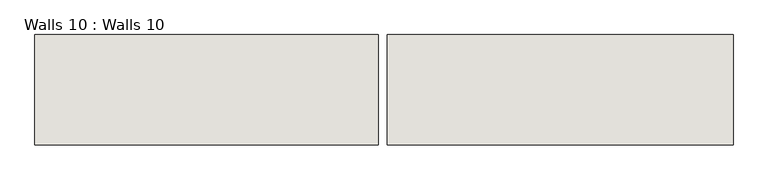
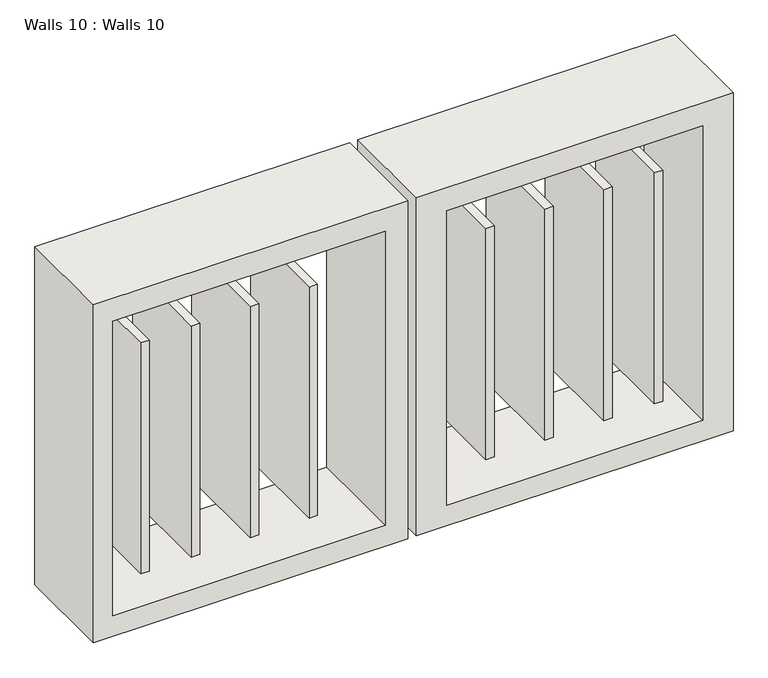
"""IFC4 building model written with IfcOpenShell, lengths in millimetres: wall geometry, Walls 10 : Walls 10."""

from ifc_helpers import new_model, si_unit, frame, origin, place, context, project, spatial, polyline, outline, extrude, source, transform, mapped, element, save


def walls_10_walls_10_47add98f(model_context):
    return source(origin(), model_context, "Body", "SweptSolid", [
        extrude(outline(polyline([(0.0, -9680.3407032), (0.0, -8731.0177942), (1078.2214623, -8731.0177942), (1078.2214623, -9680.3407032), (0.0, -9680.3407032)]), holes=[polyline([(65.8898568, -9620.7853822), (1004.6540417, -9620.7853822), (1004.6540417, -8799.2444612), (65.8898568, -8799.2444612), (65.8898568, -9620.7853822)])]), frame((0.0, 3656.1956099, 0.0), z_axis=(0.0, 1.0, 0.0), x_axis=(0.0, 0.0, 1.0)), (0.0, 0.0, 1.0), 304.8),
        extrude(outline(polyline([(0.0, -7749.9407032), (1078.2214623, -7749.9407032), (1078.2214623, -8705.6177942), (0.0, -8705.6177942), (0.0, -7749.9407032)]), holes=[polyline([(65.8898568, -8614.2962447), (1004.6540417, -8614.2962447), (1004.6540417, -7841.7447075), (65.8898568, -7841.7447075), (65.8898568, -8614.2962447)])]), frame((0.0, 3656.1956099, 0.0), z_axis=(0.0, 1.0, 0.0), x_axis=(0.0, 0.0, 1.0)), (0.0, 0.0, 1.0), 304.8),
        extrude(outline(polyline([(-9511.8500924, 3656.1956099), (-9537.2500924, 3656.1956099), (-9537.2500924, 3960.9956099), (-9511.8500924, 3960.9956099), (-9511.8500924, 3656.1956099)])), frame((0.0, 0.0, 169.6729358), z_axis=(0.0, 0.0, 1.0), x_axis=(1.0, 0.0, 0.0)), (0.0, 0.0, 1.0), 736.6),
        extrude(outline(polyline([(-9359.4500924, 3656.1956099), (-9384.8500924, 3656.1956099), (-9384.8500924, 3960.9956099), (-9359.4500924, 3960.9956099), (-9359.4500924, 3656.1956099)])), frame((0.0, 0.0, 169.6729358), z_axis=(0.0, 0.0, 1.0), x_axis=(1.0, 0.0, 0.0)), (0.0, 0.0, 1.0), 736.6),
        extrude(outline(polyline([(-9181.6500924, 3656.1956099), (-9207.0500924, 3656.1956099), (-9207.0500924, 3960.9956099), (-9181.6500924, 3960.9956099), (-9181.6500924, 3656.1956099)])), frame((0.0, 0.0, 169.6729358), z_axis=(0.0, 0.0, 1.0), x_axis=(1.0, 0.0, 0.0)), (0.0, 0.0, 1.0), 736.6),
        extrude(outline(polyline([(-9003.8500924, 3656.1956099), (-9029.2500924, 3656.1956099), (-9029.2500924, 3960.9956099), (-9003.8500924, 3960.9956099), (-9003.8500924, 3656.1956099)])), frame((0.0, 0.0, 169.6729358), z_axis=(0.0, 0.0, 1.0), x_axis=(1.0, 0.0, 0.0)), (0.0, 0.0, 1.0), 736.6),
        extrude(outline(polyline([(-8470.4500924, 3656.1956099), (-8495.8500924, 3656.1956099), (-8495.8500924, 3960.9956099), (-8470.4500924, 3960.9956099), (-8470.4500924, 3656.1956099)])), frame((0.0, 0.0, 169.6729358), z_axis=(0.0, 0.0, 1.0), x_axis=(1.0, 0.0, 0.0)), (0.0, 0.0, 1.0), 736.6),
        extrude(outline(polyline([(-8292.6500924, 3656.1956099), (-8318.0500924, 3656.1956099), (-8318.0500924, 3960.9956099), (-8292.6500924, 3960.9956099), (-8292.6500924, 3656.1956099)])), frame((0.0, 0.0, 169.6729358), z_axis=(0.0, 0.0, 1.0), x_axis=(1.0, 0.0, 0.0)), (0.0, 0.0, 1.0), 736.6),
        extrude(outline(polyline([(-8114.8500924, 3656.1956099), (-8140.2500924, 3656.1956099), (-8140.2500924, 3960.9956099), (-8114.8500924, 3960.9956099), (-8114.8500924, 3656.1956099)])), frame((0.0, 0.0, 169.6729358), z_axis=(0.0, 0.0, 1.0), x_axis=(1.0, 0.0, 0.0)), (0.0, 0.0, 1.0), 736.6),
        extrude(outline(polyline([(-7962.4500924, 3656.1956099), (-7987.8500924, 3656.1956099), (-7987.8500924, 3960.9956099), (-7962.4500924, 3960.9956099), (-7962.4500924, 3656.1956099)])), frame((0.0, 0.0, 169.6729358), z_axis=(0.0, 0.0, 1.0), x_axis=(1.0, 0.0, 0.0)), (0.0, 0.0, 1.0), 736.6),
    ])


if __name__ == "__main__":
    model = new_model("IFC4")
    model_context = context("Model", 3, world=origin())
    ifc_project = project(units=[si_unit("LENGTHUNIT", "METRE", prefix="MILLI")], contexts=[model_context])
    site = spatial("IfcSite", under=ifc_project)
    building = spatial("IfcBuilding", under=site)
    placement = place(None, origin())
    walls_10_walls_10_shape = walls_10_walls_10_47add98f(model_context)
    element("IfcWall", 1, ObjectType="Walls 10 : Walls 10", at=placement, inside=building, context=model_context, shape_type="MappedRepresentation", body=[
        mapped(walls_10_walls_10_shape, transform((0.0, 0.0, 0.0), x_axis=(1.0, 0.0, 0.0), y_axis=(0.0, 1.0, 0.0), z_axis=(0.0, 0.0, 1.0))),
    ])
    save(model, "model.ifc")

# Revit data of these elements
# Element 1 (IfcWall, "Walls 10 : Walls 10")
#   Materials on its faces: "Default Wall"
# Materials
#   "Default Wall": colour RGB 80 80 80, transparency 0
